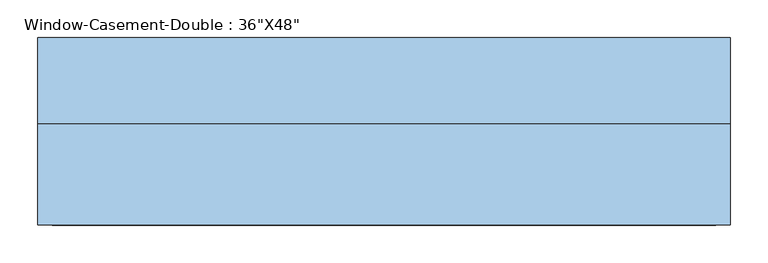
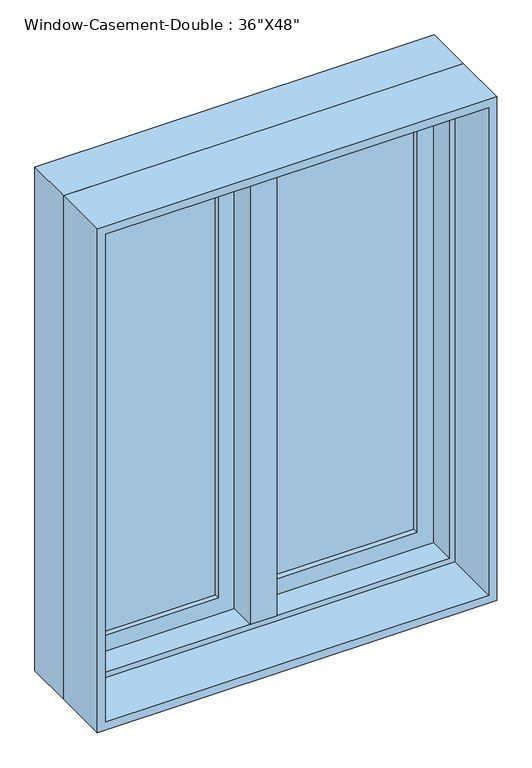
"""IFC4 building model written with IfcOpenShell, lengths in millimetres: window geometry."""

from ifc_helpers import new_model, si_unit, frame, origin, place, context, project, spatial, polyline, outline, extrude, faceted_brep, source, transform, mapped, element, save


def window_d341e8ac(model_context):
    return source(origin(), model_context, "Body", "SolidModel", [
        faceted_brep([(9.525, 133.35, 2120.9), (-9.525, 133.35, 2120.9), (-9.525, 82.55, 2120.9), (9.525, 82.55, 2120.9), (9.525, 133.35, 927.1), (9.525, 82.55, 927.1), (-9.525, 82.55, 927.1), (-9.525, 133.35, 927.1), (-9.525, 82.55, 946.15), (-9.525, 82.55, 2101.85), (-30.1625, 82.55, 946.15), (-30.1625, 82.55, 2101.85), (-30.1625, 19.05, 946.15), (-30.1625, 19.05, 2101.85), (30.1625, 19.05, 946.15), (30.1625, 19.05, 2101.85), (30.1625, 82.55, 946.15), (30.1625, 82.55, 2101.85), (9.525, 82.55, 946.15), (9.525, 82.55, 2101.85)], [[[0, 1, 2, 3]], [[4, 5, 6, 7]], [[1, 0, 4, 7]], [[2, 1, 7, 6, 8, 9]], [[9, 8, 10, 11]], [[11, 10, 12, 13]], [[13, 12, 14, 15]], [[15, 14, 16, 17]], [[17, 16, 18, 19]], [[0, 3, 19, 18, 5, 4]], [[18, 8, 6, 5]], [[9, 19, 3, 2]], [[8, 18, 16, 14, 12, 10]], [[19, 9, 11, 13, 15, 17]]]),
        extrude(outline(polyline([(-66.675, 114.3), (-66.675, 107.95), (-387.35, 107.95), (-387.35, 114.3), (-66.675, 114.3)])), frame((0.0, 0.0, 984.25), z_axis=(0.0, 0.0, 1.0), x_axis=(1.0, 0.0, 0.0)), (0.0, 0.0, 1.0), 1079.5),
        extrude(outline(polyline([(-387.35, 95.25), (-387.35, 101.6), (-66.675, 101.6), (-66.675, 95.25), (-387.35, 95.25)])), frame((0.0, 0.0, 984.25), z_axis=(0.0, 0.0, 1.0), x_axis=(1.0, 0.0, 0.0)), (0.0, 0.0, 1.0), 1079.5),
        extrude(outline(polyline([(387.35, 114.3), (387.35, 107.95), (66.675, 107.95), (66.675, 114.3), (387.35, 114.3)])), frame((0.0, 0.0, 984.25), z_axis=(0.0, 0.0, 1.0), x_axis=(1.0, 0.0, 0.0)), (0.0, 0.0, 1.0), 1079.5),
        extrude(outline(polyline([(66.675, 95.25), (66.675, 101.6), (387.35, 101.6), (387.35, 95.25), (66.675, 95.25)])), frame((0.0, 0.0, 984.25), z_axis=(0.0, 0.0, 1.0), x_axis=(1.0, 0.0, 0.0)), (0.0, 0.0, 1.0), 1079.5),
        extrude(outline(polyline([(2120.9, -444.5), (927.1, -444.5), (927.1, -9.525), (2120.9, -9.525), (2120.9, -444.5)]), holes=[polyline([(2063.75, -66.675), (984.25, -66.675), (984.25, -387.35), (2063.75, -387.35), (2063.75, -66.675)])]), frame((0.0, 82.55, 0.0), z_axis=(0.0, 1.0, 0.0), x_axis=(0.0, 0.0, 1.0)), (0.0, 0.0, 1.0), 44.45),
        extrude(outline(polyline([(927.1, 444.5), (2120.9, 444.5), (2120.9, 9.525), (927.1, 9.525), (927.1, 444.5)]), holes=[polyline([(984.25, 66.675), (2063.75, 66.675), (2063.75, 387.35), (984.25, 387.35), (984.25, 66.675)])]), frame((0.0, 82.55, 0.0), z_axis=(0.0, 1.0, 0.0), x_axis=(0.0, 0.0, 1.0)), (0.0, 0.0, 1.0), 44.45),
        extrude(outline(polyline([(2133.6, -457.2), (914.4, -457.2), (914.4, 457.2), (2133.6, 457.2), (2133.6, -457.2)]), holes=[polyline([(2114.55, 438.15), (933.45, 438.15), (933.45, -438.15), (2114.55, -438.15), (2114.55, 438.15)])]), frame((0.0, -114.3, 0.0), z_axis=(0.0, 1.0, 0.0), x_axis=(0.0, 0.0, 1.0)), (0.0, 0.0, 1.0), 133.35),
        faceted_brep([(425.45, 82.55, 2101.85), (425.45, 19.05, 2101.85), (-425.45, 19.05, 2101.85), (-425.45, 82.55, 2101.85), (444.5, 133.35, 2120.9), (444.5, 82.55, 2120.9), (-444.5, 82.55, 2120.9), (-444.5, 133.35, 2120.9), (457.2, 19.05, 2133.6), (457.2, 133.35, 2133.6), (-457.2, 133.35, 2133.6), (-457.2, 19.05, 2133.6), (-425.45, 19.05, 946.15), (-425.45, 82.55, 946.15), (-444.5, 82.55, 927.1), (-444.5, 133.35, 927.1), (-457.2, 133.35, 914.4), (-457.2, 19.05, 914.4), (425.45, 19.05, 946.15), (425.45, 82.55, 946.15), (444.5, 82.55, 927.1), (444.5, 133.35, 927.1), (457.2, 133.35, 914.4), (457.2, 19.05, 914.4)], [[[0, 1, 2, 3]], [[4, 5, 6, 7]], [[8, 9, 10, 11]], [[3, 2, 12, 13]], [[7, 6, 14, 15]], [[11, 10, 16, 17]], [[13, 12, 18, 19]], [[15, 14, 20, 21]], [[17, 16, 22, 23]], [[11, 17, 23, 8], [1, 18, 12, 2]], [[19, 18, 1, 0]], [[5, 20, 14, 6], [3, 13, 19, 0]], [[21, 20, 5, 4]], [[23, 22, 9, 8]], [[9, 22, 16, 10], [7, 15, 21, 4]]]),
    ])


if __name__ == "__main__":
    model = new_model("IFC4")
    model_context = context("Model", 3, world=origin())
    ifc_project = project(units=[si_unit("LENGTHUNIT", "METRE", prefix="MILLI")], contexts=[model_context])
    site = spatial("IfcSite", under=ifc_project)
    building = spatial("IfcBuilding", under=site)
    placement = place(None, origin())
    window_shape = window_d341e8ac(model_context)
    element("IfcWindow", 1, ObjectType="Window-Casement-Double : 36\"X48\"", at=placement, inside=building, context=model_context, shape_type="MappedRepresentation", body=[
        mapped(window_shape, transform((0.0, 0.0, 0.0), x_axis=(1.0, 0.0, 0.0), y_axis=(0.0, 1.0, 0.0), z_axis=(0.0, 0.0, 1.0))),
    ])
    save(model, "model.ifc")

# Revit data of these elements
# Type "Window-Casement-Double : 36\"X48\""
#   Type Mark = "21"
#   Fire Rating = "0.5h"
#   Assembly Code = "B2020100"
#   Analytic Construction = "Double glazing - domestic"
#   Frame Extension [instance default] = 0' - 0 1/4"
#   Window Inset [instance default] = 0' - 0"
#   Wall Thickness [instance default] = 0' - 6"
#   Interior Wall Closure [instance default] = 0' - 2 1/4"
#   Half Width = 1' - 6"
#   Visual Light Transmittance = 0.81
#   Thermal Resistance (R) = 1.8146 (h·ft²·°F)/BTU
#   Solar Heat Gain Coefficient = 0.76
#   Rough Width = 3' - 0 1/2"
#   Rough Height = 4' - 0 1/2"
#   Height = 4' - 0"
#   Heat Transfer Coefficient (U) = 0.5511 BTU/(h·ft²·°F)
#   Exterior Wall Closure [instance default] = 0' - 1 1/4"
#   Extension Jamb [instance default] = 0' - 2 1/4"
#   Default Sill Height = 3' - 0"
#   Width = 3' - 0"
#   Muntin Visibility = yes
#   Interior Trim Visibility [instance default] = yes
#   Exterior Trim Visibility [instance default] = yes
#   Extension Jamb Visibility [instance default] = yes
#   Interior Trim Material = Wood - Stained
#   Muntin Pattern = Muntin Pattern_2x2 : Muntin Pattern_2x2
#   Interior Trim = Trim-Window-Interior-Flat : Picture Frame
#   Interior Frame Material = Wood - Stained
#   Glass Panel Material = Glass
#   Exterior Trim Material = Clad - White
#   Exterior Trim = Trim-Window-Exterior-Flat : with Sill
#   Exterior Frame Material = Clad - White
#   Wall Closure = (empty or 0)
# Element 1 (IfcWindow, "Window-Casement-Double : 36\"X48\"")
#   Wall Thickness = 0' - 9"
#   Extension Jamb = 0' - 5 1/4"
#   Materials on its faces: "Wood - Stained", "Glass", "Clad - White"
# Materials
#   "Wood - Stained": class "Wood", colour RGB 224 178 126, transparency 0, Cost = 0
#   "Glass": class "Glass", colour RGB 0 128 192, transparency 0.75, Description = "Soda Lime Glass", Cost = 0
#   "Clad - White": class "Wood", colour RGB 242 242 238, transparency 0, Cost = 0
